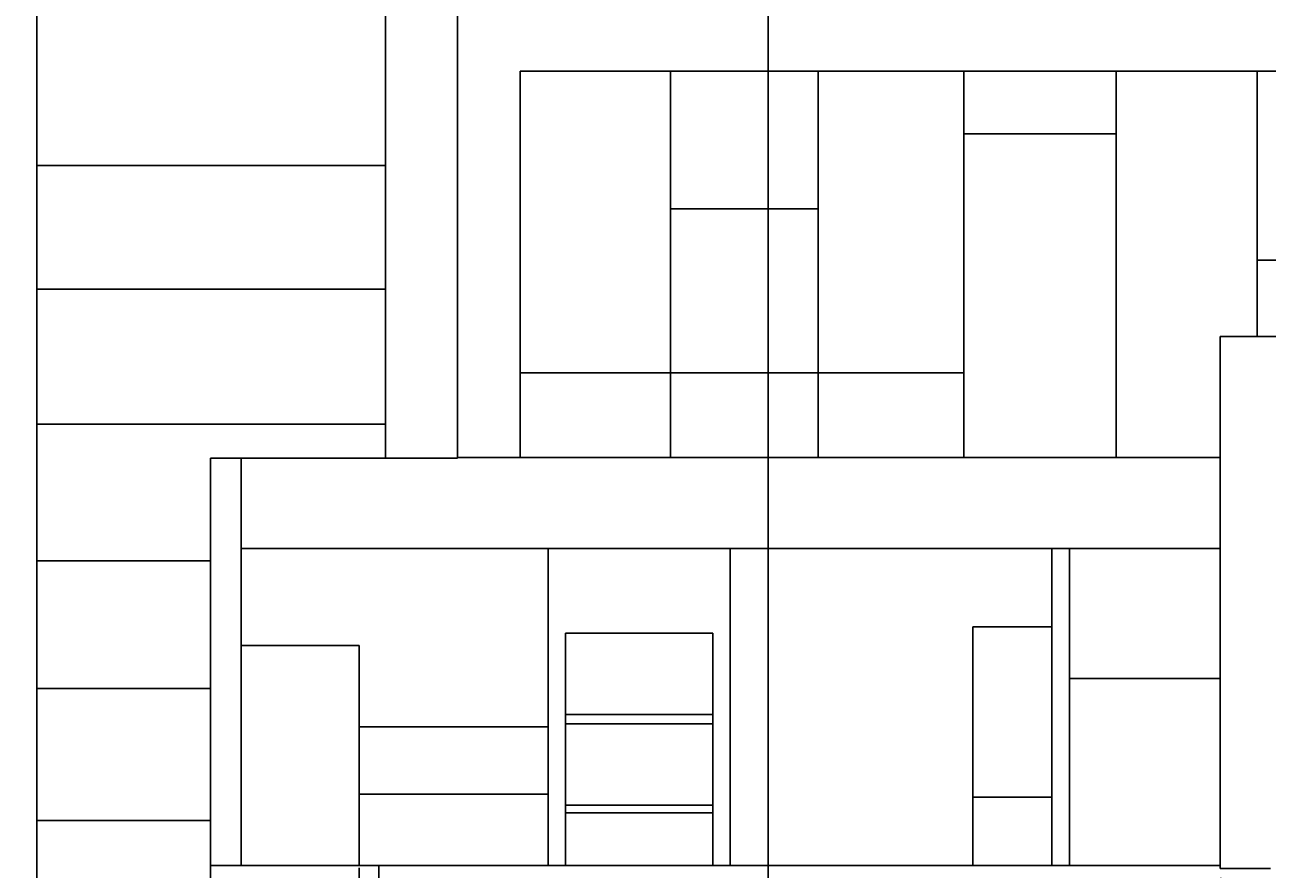
# Model space of a CAD drawing. Units: inches. Extents: x -117 to 121, y -77 to 40.
# Tile 27 of 45: x -23 to 9, y -8 to 14. Entities that reach past the tile are written whole.
import ezdxf

# ---------------------------------------------------------------- set-up
doc = ezdxf.new("R2010")
doc.units = ezdxf.units.IN
doc.header["$MEASUREMENT"] = 0
doc.layers.add('A-ANNO-DIMS', color=2, linetype='Continuous', lineweight=18)
doc.layers.add('A-ELEV', color=7, linetype='Continuous', lineweight=25)
doc.styles.get("Standard").update_dxf_attribs({"font": 'arial.ttf'})
doc.dimstyles.get("Standard").update_dxf_attribs({"dimtxt": 0.18, "dimasz": 0.18, "dimexe": 0.18, "dimexo": 0.0625, "dimgap": 0.09, "dimtad": 0, "dimtih": 1, "dimtoh": 1, "dimdec": 4, "dimzin": 0, "dimdsep": 46, "dimtxsty": 'Standard', "dimcen": 0.09, "dimadec": 0, "dimazin": 0, "dimtfac": 1, "dimtdec": 4, "dimtofl": 0, "dimtmove": 0, "dimatfit": 3, "dimfxl": 1, "dimtolj": 1, "dimtzin": 0, "dimarcsym": 0})

# ---------------------------------------------------------------- blocks, each defined once
blk = doc.blocks.new('*D13')
at = {"layer": 'A-ANNO-DIMS', "color": 0, "lineweight": -2, "transparency": 16777216}
for p, q in [((-2.663, 27.063), (-117.024, 27.063)), ((-116.844, 26.883), (-116.844, -16.974)), ((-116.844, -61.196), (-116.844, -17.338)), ((-106.096, -61.376), (-117.024, -61.376))]:
    blk.add_line(p, q, dxfattribs=at)
at = {"layer": 'A-ANNO-DIMS', "color": 0, "transparency": 16777216}
for points in [[(-116.874, 26.883), (-116.814, 26.883), (-116.844, 27.063)], [(-116.874, -61.196), (-116.814, -61.196), (-116.844, -61.376)]]:
    blk.add_solid(points, dxfattribs=at)
at = {"layer": 'Defpoints', "color": 0, "transparency": 16777216}
for p in [(-2.6, 27.063), (-116.844, -61.376), (-106.034, -61.376)]:
    blk.add_point(p, dxfattribs=at)
at = {"layer": 'A-ANNO-DIMS', "color": 0, "transparency": 16777216, "insert": (-116.844, -17.156), "char_height": 0.18, "attachment_point": 5}
blk.add_mtext('\\A1;88.44', dxfattribs=at)
blk = doc.blocks.new('*D22')
at = {"layer": 'A-ANNO-DIMS', "color": 0, "lineweight": -2, "transparency": 16777216}
for p, q in [((-23.864, 8.087), (-23.864, 38.61)), ((-2.6, 27.126), (-2.6, 38.61)), ((-23.684, 38.43), (-13.697, 38.43)), ((-2.78, 38.43), (-12.767, 38.43))]:
    blk.add_line(p, q, dxfattribs=at)
at = {"layer": 'A-ANNO-DIMS', "color": 0, "transparency": 16777216}
for points in [[(-23.684, 38.46), (-23.684, 38.4), (-23.864, 38.43)], [(-2.78, 38.46), (-2.78, 38.4), (-2.6, 38.43)]]:
    blk.add_solid(points, dxfattribs=at)
at = {"layer": 'Defpoints', "color": 0, "transparency": 16777216}
for p in [(-2.6, 38.43), (-2.6, 27.063), (-23.864, 8.025)]:
    blk.add_point(p, dxfattribs=at)
at = {"layer": 'A-ANNO-DIMS', "color": 0, "transparency": 16777216, "insert": (-13.232, 38.43), "char_height": 0.18, "attachment_point": 5}
blk.add_mtext('\\A1;21.264', dxfattribs=at)
blk = doc.blocks.new('*D32')
at = {"layer": 'A-ANNO-DIMS', "color": 0, "lineweight": -2, "transparency": 16777216}
for p, q in [((-3.85, -45.55), (-3.85, 38.61)), ((20.293, -45.55), (20.293, 38.61)), ((-3.67, 38.43), (7.757, 38.43)), ((20.113, 38.43), (8.686, 38.43))]:
    blk.add_line(p, q, dxfattribs=at)
at = {"layer": 'A-ANNO-DIMS', "color": 0, "transparency": 16777216}
for points in [[(-3.67, 38.46), (-3.67, 38.4), (-3.85, 38.43)], [(20.113, 38.46), (20.113, 38.4), (20.293, 38.43)]]:
    blk.add_solid(points, dxfattribs=at)
at = {"layer": 'Defpoints', "color": 0, "transparency": 16777216}
for p in [(20.293, 38.43), (-3.85, -45.613), (20.293, -45.613)]:
    blk.add_point(p, dxfattribs=at)
at = {"layer": 'A-ANNO-DIMS', "color": 0, "transparency": 16777216, "insert": (8.222, 38.43), "char_height": 0.18, "attachment_point": 5}
blk.add_mtext('\\A1;24.142', dxfattribs=at)
blk = doc.blocks.new('*D56')
at = {"layer": 'A-ANNO-DIMS', "color": 0, "lineweight": -2, "transparency": 16777216}
for p, q in [((-14.23, -7.853), (-14.23, -77.193)), ((7.628, -8.105), (7.628, -77.193)), ((-14.05, -77.013), (-3.766, -77.013)), ((7.448, -77.013), (-2.835, -77.013))]:
    blk.add_line(p, q, dxfattribs=at)
at = {"layer": 'A-ANNO-DIMS', "color": 0, "transparency": 16777216}
for points in [[(-14.05, -76.983), (-14.05, -77.043), (-14.23, -77.013)], [(7.448, -76.983), (7.448, -77.043), (7.628, -77.013)]]:
    blk.add_solid(points, dxfattribs=at)
at = {"layer": 'Defpoints', "color": 0, "transparency": 16777216}
for p in [(-14.23, -7.791), (7.628, -8.042), (7.628, -77.013)]:
    blk.add_point(p, dxfattribs=at)
at = {"layer": 'A-ANNO-DIMS', "color": 0, "transparency": 16777216, "insert": (-3.301, -77.013), "char_height": 0.18, "attachment_point": 5}
blk.add_mtext('\\A1;21.858', dxfattribs=at)

msp = doc.modelspace()

# ---------------------------------------------------------------- linework, layer by layer
at = {"layer": 'A-ELEV'}
for p, q in [((-22.4056, 14.0735), (-22.4056, -14.3771)), ((-13.5598, 14.0735), (-13.5598, 2.5407)), ((-11.738, 14.0735), (-11.738, 2.5577)), ((12.1837, 12.3611), (-10.1416, 12.3611)), ((-10.1416, 12.3611), (-10.1416, 2.5577)), ((-6.3314, 12.3611), (-6.3314, 2.5577)), ((-2.5808, 12.3611), (-2.5808, 2.5577)), ((1.1103, 12.3611), (1.1103, 2.5577)), ((4.98, 12.3611), (4.98, 2.5577)), ((8.5521, 12.3611), (8.5521, 5.6236)), ((1.1103, 10.7702), (4.98, 10.7702)), ((-22.4056, 9.962), (-13.5598, 9.962)), ((-6.3314, 8.8674), (-2.5808, 8.8674)), ((8.5521, 7.5594), (12.1837, 7.5594)), ((-22.4056, 6.8303), (-13.5598, 6.8303)), ((7.6115, 2.5577), (7.6115, 5.6237)), ((7.6115, 5.6237), (13.9784, 5.623)), ((-10.1416, 4.705), (1.1103, 4.705)), ((-22.4056, 3.4006), (-13.5598, 3.4006)), ((-18.0037, 2.5407), (-11.738, 2.5407)), ((-18.0037, 2.5407), (-18.0037, -7.7907)), ((-17.2198, 2.5407), (-17.2198, -7.7907)), ((-10.1416, 2.5577), (-11.738, 2.5577)), ((-10.1416, 2.5577), (7.6115, 2.5577)), ((7.6115, 2.5577), (7.6115, -7.8658)), ((-17.2198, 0.2476), (7.6115, 0.2476)), ((-9.4355, 0.2476), (-9.4355, -7.7907)), ((-4.8155, 0.2476), (-4.8155, -7.7907)), ((3.3485, 0.2476), (3.3485, -7.7907)), ((3.7915, 0.2476), (3.7915, -7.7907)), ((-22.4056, -0.0626), (-18.0037, -0.0626)), ((1.3367, -1.7403), (1.3367, -7.7907)), ((3.3485, -1.7403), (1.3367, -1.7403)), ((-8.9925, -1.8989), (-8.9925, -7.7907)), ((-8.9925, -1.8989), (-5.2585, -1.8989)), ((-5.2585, -1.8989), (-5.2585, -7.7907)), ((-17.2198, -2.2136), (-14.2298, -2.2136)), ((-14.2298, -2.2136), (-14.2298, -7.7907)), ((3.7915, -3.0486), (7.6115, -3.0486)), ((-22.4056, -3.3034), (-18.0037, -3.3034)), ((-8.9925, -3.9605), (-5.2585, -3.9605)), ((-14.2298, -4.2786), (-9.4355, -4.2786)), ((-8.9925, -4.1983), (-5.2585, -4.1983)), ((-14.2298, -5.9834), (-9.4355, -5.9834)), ((-8.9925, -6.2599), (-5.2585, -6.2599)), ((1.3367, -6.0616), (3.3485, -6.0616)), ((-8.9925, -6.4581), (-5.2585, -6.4581)), ((-22.4056, -6.6545), (-18.0037, -6.6545)), ((-18.0037, -7.7907), (7.6115, -7.7907)), ((-18.0037, -7.7907), (-18.0037, -14.3771)), ((-13.7272, -8.6912), (-13.7272, -7.7907)), ((7.6115, -7.8658), (8.8925, -7.8658))]:
    msp.add_line(p, q, dxfattribs=at)

# ---------------------------------------------------------------- dimensions: what is measured, and where the dimension line sits
at = {"layer": 'A-ANNO-DIMS'}
for base, p1, p2, picture, middle in [((-2.6001, 38.4297), (-23.8637, 8.0246), (-2.6001, 27.0634), '*D22', (-13.2319, 38.4297)), ((20.2929, 38.4297), (-3.8495, -45.6125), (20.2929, -45.6125), '*D32', (8.2217, 38.4297)), ((7.6284, -77.0135), (-14.2298, -7.7907), (7.6284, -8.0421), '*D56', (-3.3007, -77.0135))]:
    dim = msp.add_linear_dim(base=base, p1=p1, p2=p2, dimstyle='Standard', override={"dimdec": 3, "dimlfac": 1, "dimrnd": 0, "dimzin": 0, "dimdsep": 46, "dimlunit": 2}, dxfattribs=at)
    dim.commit()
    dim.dimension.update_dxf_attribs({"geometry": picture, "text_midpoint": middle})
dim = msp.add_linear_dim(base=(-116.8438, -61.3756), p1=(-2.6001, 27.0634), p2=(-106.0338, -61.3756), angle=90, dimstyle='Standard', override={"dimdec": 2, "dimlfac": 1, "dimrnd": 0, "dimzin": 0, "dimdsep": 46, "dimlunit": 2}, dxfattribs=at)
dim.commit()
dim.dimension.update_dxf_attribs({"geometry": '*D13', "text_midpoint": (-116.8438, -17.1561)})

doc.saveas('drawing.dxf')
